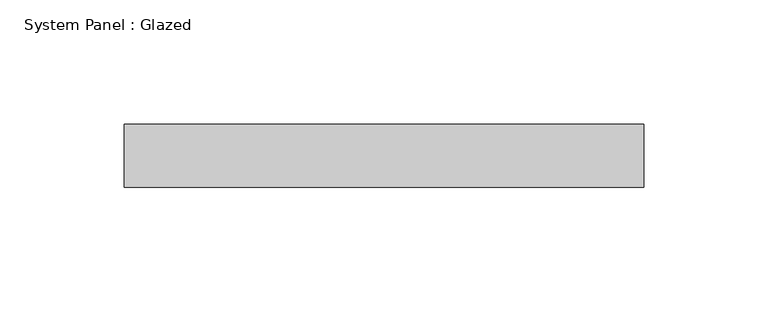
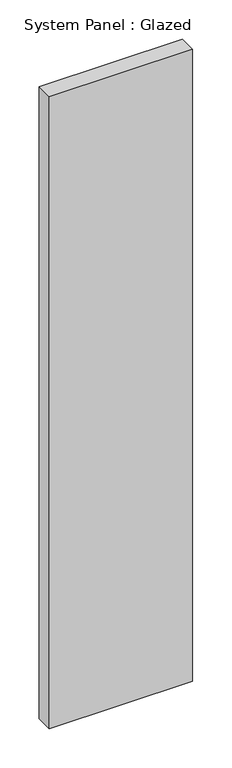
"""IFC4 building model written with IfcOpenShell, lengths in millimetres: plate geometry, System Panel : Glazed."""

from ifc_helpers import new_model, si_unit, origin, origin_with_axes, place, context, project, spatial, polyline, outline, extrude, source, transform, mapped, element, save


def system_panel_glazed_1899ac7a(model_context):
    return source(origin(), model_context, "Body", "SweptSolid", [
        extrude(outline(polyline([(104.775, 19.05), (-104.775, 19.05), (-104.775, 44.45), (104.775, 44.45), (104.775, 19.05)])), origin_with_axes(), (0.0, 0.0, 1.0), 977.9),
    ])


if __name__ == "__main__":
    model = new_model("IFC4")
    model_context = context("Model", 3, world=origin())
    ifc_project = project(units=[si_unit("LENGTHUNIT", "METRE", prefix="MILLI")], contexts=[model_context])
    site = spatial("IfcSite", under=ifc_project)
    building = spatial("IfcBuilding", under=site)
    placement = place(None, origin())
    system_panel_glazed_shape = system_panel_glazed_1899ac7a(model_context)
    element("IfcPlate", 1, ObjectType="System Panel : Glazed", at=placement, inside=building, context=model_context, shape_type="MappedRepresentation", body=[
        mapped(system_panel_glazed_shape, transform((0.0, 0.0, 0.0), x_axis=(1.0, 0.0, 0.0), y_axis=(0.0, 1.0, 0.0), z_axis=(0.0, 0.0, 1.0))),
    ])
    save(model, "model.ifc")

# Revit data of these elements
# Type "System Panel : Glazed"
#   Construction Type Id = "GSP4R"
#   Analytic Construction = "1/8 in Pilkington single glazing"
#   Visual Light Transmittance = 0.9
#   Solar Heat Gain Coefficient = 0.86
#   Heat Transfer Coefficient (U) = 1.18115 BTU/(h·ft²·°F)
#   Define Thermal Properties by = 1
# Element 1 (IfcPlate, "System Panel : Glazed")
#   Materials on its faces: "Glass"
# Materials
#   "Glass": class "Glass", colour RGB 0 128 192, transparency 0.75, Description = "Soda Lime Glass", Cost = 0
